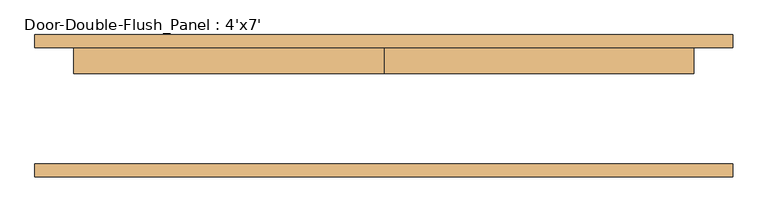
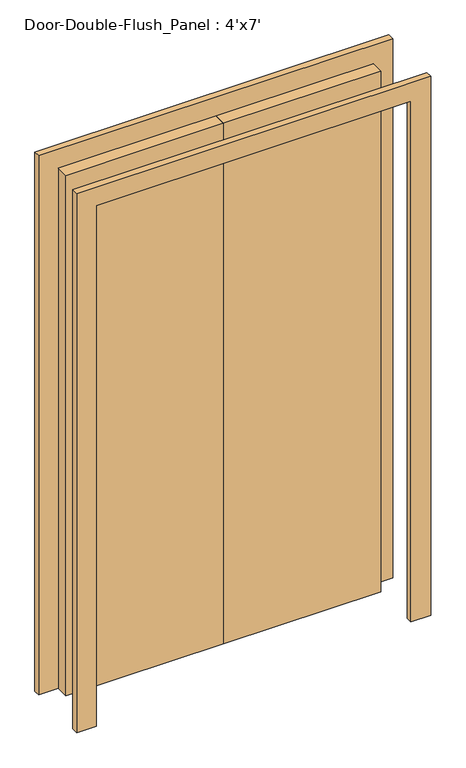
"""IFC4 building model written with IfcOpenShell, lengths in millimetres: door geometry, Door-Double-Flush_Panel : 4'x7'."""

from ifc_helpers import new_model, si_unit, frame, origin, origin_with_axes, place, context, project, spatial, polyline, outline, extrude, source, transform, mapped, element, save


def door_double_flush_panel_4_x7_7c704b5a(model_context):
    return source(origin(), model_context, "Body", "SweptSolid", [
        extrude(outline(polyline([(2133.6, -609.6), (2133.6, 609.6), (0.0, 609.6), (0.0, 685.8), (2209.8, 685.8), (2209.8, -685.8), (0.0, -685.8), (0.0, -609.6), (2133.6, -609.6)])), frame((0.0, 114.3, 0.0), z_axis=(0.0, 1.0, 0.0), x_axis=(0.0, 0.0, 1.0)), (0.0, 0.0, 1.0), 25.4),
        extrude(outline(polyline([(2133.6, -609.6), (2133.6, 609.6), (0.0, 609.6), (0.0, 685.8), (2209.8, 685.8), (2209.8, -685.8), (0.0, -685.8), (0.0, -609.6), (2133.6, -609.6)])), frame((0.0, -139.7, 0.0), z_axis=(0.0, 1.0, 0.0), x_axis=(0.0, 0.0, 1.0)), (0.0, 0.0, 1.0), 25.4),
        extrude(outline(polyline([(-609.6, 114.3), (0.0, 114.3), (0.0, 63.5), (-609.6, 63.5), (-609.6, 114.3)])), origin_with_axes(), (0.0, 0.0, 1.0), 2133.6),
        extrude(outline(polyline([(0.0, 114.3), (609.6, 114.3), (609.6, 63.5), (0.0, 63.5), (0.0, 114.3)])), origin_with_axes(), (0.0, 0.0, 1.0), 2133.6),
    ])


if __name__ == "__main__":
    model = new_model("IFC4")
    model_context = context("Model", 3, world=origin())
    ifc_project = project(units=[si_unit("LENGTHUNIT", "METRE", prefix="MILLI")], contexts=[model_context])
    site = spatial("IfcSite", under=ifc_project)
    building = spatial("IfcBuilding", under=site)
    placement = place(None, origin())
    door_double_flush_panel_4_x7_shape = door_double_flush_panel_4_x7_7c704b5a(model_context)
    element("IfcDoor", 1, ObjectType="Door-Double-Flush_Panel : 4'x7'", at=placement, inside=building, context=model_context, shape_type="MappedRepresentation", body=[
        mapped(door_double_flush_panel_4_x7_shape, transform((0.0, 0.0, 0.0), x_axis=(1.0, 0.0, 0.0), y_axis=(0.0, 1.0, 0.0), z_axis=(0.0, 0.0, 1.0))),
    ])
    save(model, "model.ifc")

# Revit data of these elements
# Type "Door-Double-Flush_Panel : 4'x7'"
#   Type Mark = "9"
#   Construction Type Id = "DOOR"
#   Assembly Code = "C1020"
#   Analytic Construction = "Wooden"
#   Thickness = 0' - 2"
#   Thermal Resistance (R) = 2.5876 (h·ft²·°F)/BTU
#   Swing Angle [instance default] = 90.00°
#   Panel Width = 2' - 0"
#   Heat Transfer Coefficient (U) = 0.3865 BTU/(h·ft²·°F)
#   Height = 7' - 0"
#   Trim Projection Ext = 0' - 1"
#   Trim Projection Int = 0' - 1"
#   Trim Width = 0' - 3"
#   Width = 4' - 0"
#   Define Thermal Properties by = 1
#   Panel Material = Wood - Birch - Solid Stained Light Low Gloss
#   Trim Material = Paint - Sienna
#   Visual Light Transmittance = 0
#   Solar Heat Gain Coefficient = 0
#   Function = (empty or 0)
#   Wall Closure = (empty or 0)
# Element 1 (IfcDoor, "Door-Double-Flush_Panel : 4'x7'")
#   Materials on its faces: "Paint - Sienna", "Wood - Birch - Solid Stained Light Low Gloss"
# Materials
#   "Wood - Birch - Solid Stained Light Low Gloss": class "Wood", colour RGB 210 159 95, transparency 0, Cost = 0
#   "Paint - Sienna": colour RGB 118 70 51, transparency 0, Cost = 0
